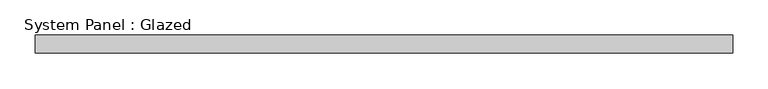
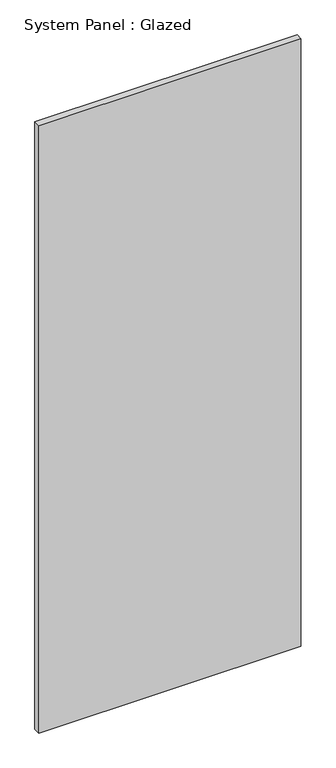
"""IFC4 building model written with IfcOpenShell, lengths in millimetres: plate geometry, System Panel : Glazed."""

from ifc_helpers import new_model, si_unit, origin, origin_with_axes, place, context, project, spatial, polyline, outline, extrude, source, transform, mapped, element, save


def system_panel_glazed_4d5331aa(model_context):
    return source(origin(), model_context, "Body", "SweptSolid", [
        extrude(outline(polyline([(492.125, 19.05), (-492.125, 19.05), (-492.125, 44.45), (492.125, 44.45), (492.125, 19.05)])), origin_with_axes(), (0.0, 0.0, 1.0), 2411.6388159),
    ])


if __name__ == "__main__":
    model = new_model("IFC4")
    model_context = context("Model", 3, world=origin())
    ifc_project = project(units=[si_unit("LENGTHUNIT", "METRE", prefix="MILLI")], contexts=[model_context])
    site = spatial("IfcSite", under=ifc_project)
    building = spatial("IfcBuilding", under=site)
    placement = place(None, origin())
    system_panel_glazed_shape = system_panel_glazed_4d5331aa(model_context)
    element("IfcPlate", 1, ObjectType="System Panel : Glazed", at=placement, inside=building, context=model_context, shape_type="MappedRepresentation", body=[
        mapped(system_panel_glazed_shape, transform((0.0, 0.0, 0.0), x_axis=(1.0, 0.0, 0.0), y_axis=(0.0, 1.0, 0.0), z_axis=(0.0, 0.0, 1.0))),
    ])
    save(model, "model.ifc")

# Revit data of these elements
# Type "System Panel : Glazed"
#   Construction Type Id = "GSP4R"
#   Analytic Construction = "1/8 in Pilkington single glazing"
#   Visual Light Transmittance = 0.9
#   Solar Heat Gain Coefficient = 0.86
#   Heat Transfer Coefficient (U) = 1.18115 BTU/(h·ft²·°F)
#   Define Thermal Properties by = 1
# Element 1 (IfcPlate, "System Panel : Glazed")
#   Materials on its faces: "Glass"
# Materials
#   "Glass": class "Glass", colour RGB 0 128 192, transparency 0.75, Description = "Soda Lime Glass", Cost = 0
